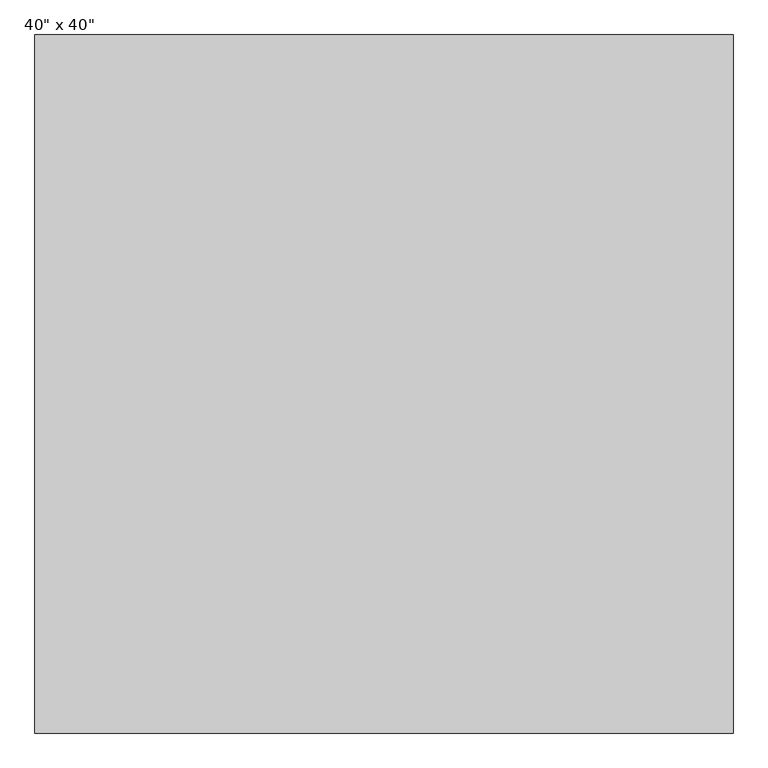
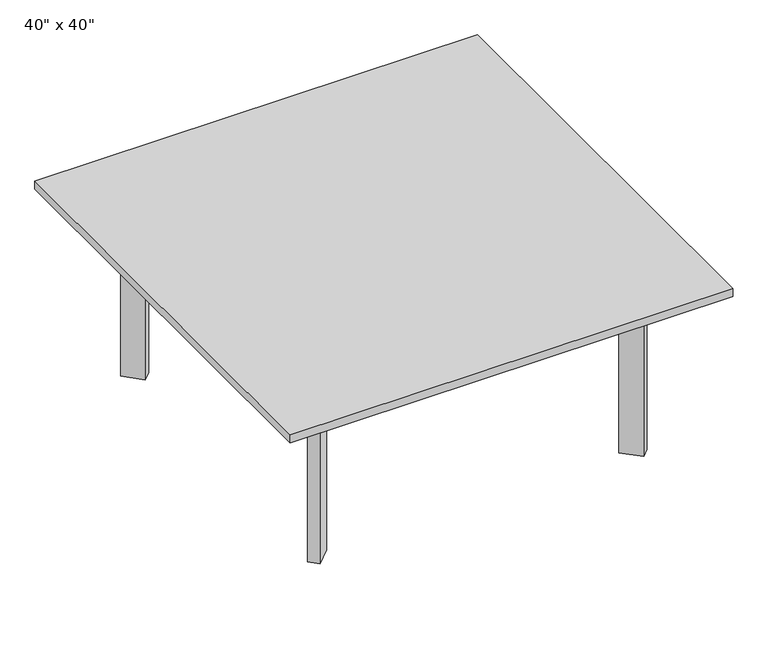
"""IFC4 building model written with IfcOpenShell, lengths in millimetres: furniture geometry."""

from ifc_helpers import new_model, si_unit, frame, origin, origin_with_axes, place, context, project, spatial, polyline, outline, extrude, source, transform, mapped, element, save


def furniture_7b9c1204(model_context):
    return source(origin(), model_context, "Body", "SweptSolid", [
        extrude(outline(polyline([(452.6196721, 448.0393443), (452.6196721, -567.9606557), (-563.3803279, -567.9606557), (-563.3803279, 448.0393443), (452.6196721, 448.0393443)])), frame((0.0, 0.0, 412.75), z_axis=(0.0, 0.0, 1.0), x_axis=(1.0, 0.0, 0.0)), (0.0, 0.0, 1.0), 19.05),
        extrude(outline(polyline([(-427.4000717, 330.0196004), (-391.4790473, 294.0985759), (-409.4395595, 276.1380637), (-445.360584, 312.0590881), (-427.4000717, 330.0196004)])), origin_with_axes(), (0.0, 0.0, 1.0), 361.95),
        extrude(outline(polyline([(316.639416, 330.0196004), (334.5999283, 312.0590881), (298.6789038, 276.1380637), (280.7183915, 294.0985759), (316.639416, 330.0196004)])), origin_with_axes(), (0.0, 0.0, 1.0), 361.95),
        extrude(outline(polyline([(334.5999283, -431.9803996), (316.639416, -449.9409119), (280.7183915, -414.0198874), (298.6789038, -396.0593751), (334.5999283, -431.9803996)])), origin_with_axes(), (0.0, 0.0, 1.0), 361.95),
        extrude(outline(polyline([(-445.360584, -431.9803996), (-409.4395595, -396.0593751), (-391.4790473, -414.0198874), (-427.4000717, -449.9409119), (-445.360584, -431.9803996)])), origin_with_axes(), (0.0, 0.0, 1.0), 361.95),
        extrude(outline(polyline([(-427.4000717, 330.0196004), (-55.3803279, -42.0001435), (316.639416, 330.0196004), (334.5999283, 312.0590881), (-37.4198156, -59.9606557), (334.5999283, -431.9803996), (316.639416, -449.9409119), (-55.3803279, -77.921168), (-427.4000717, -449.9409119), (-445.360584, -431.9803996), (-73.3408401, -59.9606557), (-445.360584, 312.0590881), (-427.4000717, 330.0196004)])), frame((0.0, 0.0, 361.95), z_axis=(0.0, 0.0, 1.0), x_axis=(1.0, 0.0, 0.0)), (0.0, 0.0, 1.0), 50.8),
    ])


if __name__ == "__main__":
    model = new_model("IFC4")
    model_context = context("Model", 3, world=origin())
    ifc_project = project(units=[si_unit("LENGTHUNIT", "METRE", prefix="MILLI")], contexts=[model_context])
    site = spatial("IfcSite", under=ifc_project)
    building = spatial("IfcBuilding", under=site)
    placement = place(None, origin())
    furniture_shape = furniture_7b9c1204(model_context)
    element("IfcFurniture", 1, ObjectType="40\" x 40\"", at=placement, inside=building, context=model_context, shape_type="MappedRepresentation", body=[
        mapped(furniture_shape, transform((0.0, 0.0, 0.0), x_axis=(1.0, 0.0, 0.0), y_axis=(0.0, 1.0, 0.0), z_axis=(0.0, 0.0, 1.0))),
    ])
    save(model, "model.ifc")

# Revit data of these elements
# Type "40\" x 40\""
#   Assembly Code = "E2020200"
#   Height = 1' - 5"
#   Length = 3' - 4"
#   Width = 3' - 4"
#   Default Elevation = 0
# Element 1 (IfcFurniture, "40\" x 40\"")
#   Materials on its faces: "Metal - Steel, Polished", "Glass - Clear, Grey"
# Materials
#   "Metal - Steel, Polished": colour RGB 57 57 57, transparency 0
#   "Glass - Clear, Grey": colour RGB 252 255 255, transparency 0.64
